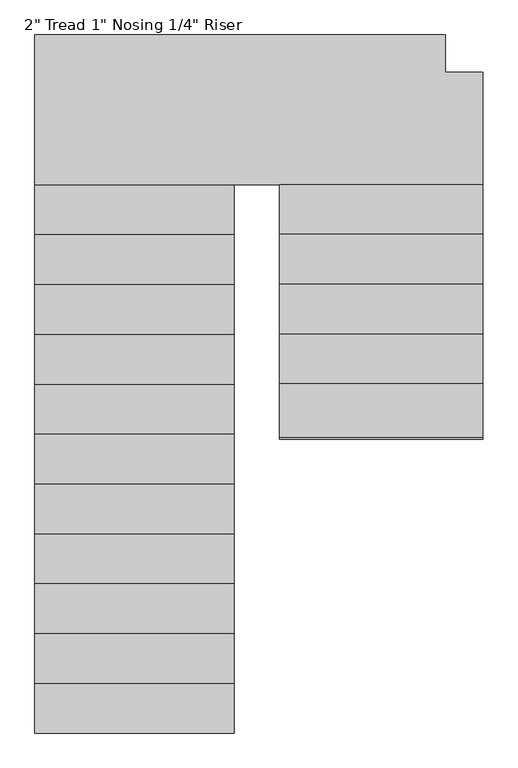
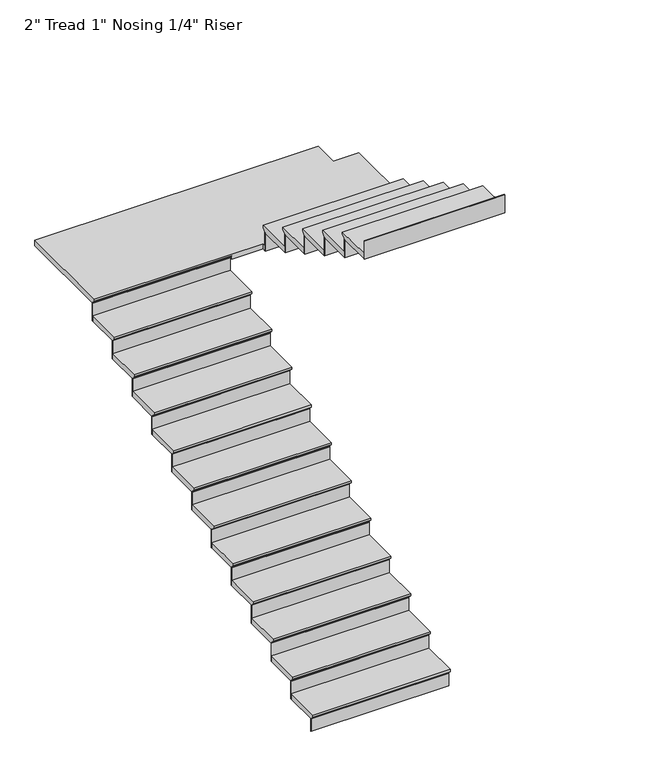
"""IFC4 building model written with IfcOpenShell, lengths in millimetres: stair flight geometry."""

from ifc_helpers import new_model, si_unit, origin, place, context, project, spatial, faceted_brep, source, transform, mapped, element, save


def stair_flight_d695bd93(model_context):
    return source(origin(), model_context, "Body", "Brep", [
        faceted_brep([(-1810.3456086, -4300.9794704, 3503.0833333), (-1810.3456086, -4300.9794704, 3522.1333333), (-3029.5456086, -4300.9794704, 3522.1333333), (-3029.5456086, -4300.9794704, 3503.0833333), (-1810.3456086, -4275.5794704, 3477.6833333), (-3029.5456086, -4275.5794704, 3477.6833333), (-1810.3456086, -3970.7794704, 3522.1333333), (-3029.5456086, -3970.7794704, 3522.1333333), (-3029.5456086, -4275.5794704, 3471.3333333), (-3029.5456086, -3970.7794704, 3471.3333333), (-1810.3456086, -3970.7794704, 3471.3333333), (-1810.3456086, -4275.5794704, 3471.3333333)], [[[0, 1, 2, 3]], [[4, 0, 3, 5]], [[2, 1, 6, 7]], [[8, 9, 10, 11]], [[2, 7, 9, 8, 5, 3]], [[8, 11, 4, 5]], [[6, 1, 0, 4, 11, 10]], [[7, 6, 10, 9]]]),
        faceted_brep([(-1810.3456086, -4275.5794704, 3471.3333333), (-1810.3456086, -4275.5794704, 3352.8), (-1810.3456086, -4269.2294704, 3352.8), (-1810.3456086, -4269.2294704, 3471.3333333), (-3029.5456086, -4275.5794704, 3471.3333333), (-3029.5456086, -4269.2294704, 3471.3333333), (-3029.5456086, -4269.2294704, 3352.8), (-3029.5456086, -4275.5794704, 3352.8)], [[[0, 1, 2, 3]], [[4, 5, 6, 7]], [[1, 0, 4, 7]], [[2, 1, 7, 6]], [[3, 2, 6, 5]], [[0, 3, 5, 4]]]),
        faceted_brep([(-1810.3456086, -3970.7794704, 3640.6666667), (-1810.3456086, -3970.7794704, 3471.3333333), (-1810.3456086, -3964.4294704, 3471.3333333), (-1810.3456086, -3964.4294704, 3640.6666667), (-3029.5456086, -3970.7794704, 3640.6666667), (-3029.5456086, -3964.4294704, 3640.6666667), (-3029.5456086, -3964.4294704, 3471.3333333), (-3029.5456086, -3970.7794704, 3471.3333333)], [[[0, 1, 2, 3]], [[4, 5, 6, 7]], [[1, 0, 4, 7]], [[2, 1, 7, 6]], [[3, 2, 6, 5]], [[0, 3, 5, 4]]]),
        faceted_brep([(-3029.5456086, -3996.1794704, 3691.4666667), (-1810.3456086, -3996.1794704, 3691.4666667), (-1810.3456086, -3665.9794704, 3691.4666667), (-3029.5456086, -3665.9794704, 3691.4666667), (-3029.5456086, -3970.7794704, 3640.6666667), (-3029.5456086, -3665.9794704, 3640.6666667), (-1810.3456086, -3665.9794704, 3640.6666667), (-1810.3456086, -3970.7794704, 3640.6666667), (-3029.5456086, -3970.7794704, 3647.0166667), (-3029.5456086, -3996.1794704, 3672.4166667), (-1810.3456086, -3970.7794704, 3647.0166667), (-1810.3456086, -3996.1794704, 3672.4166667)], [[[0, 1, 2, 3]], [[4, 5, 6, 7]], [[0, 3, 5, 4, 8, 9]], [[4, 7, 10, 8]], [[2, 1, 11, 10, 7, 6]], [[3, 2, 6, 5]], [[11, 1, 0, 9]], [[10, 11, 9, 8]]]),
        faceted_brep([(-1810.3456086, -3665.9794704, 3810.0), (-1810.3456086, -3665.9794704, 3640.6666667), (-1810.3456086, -3659.6294704, 3640.6666667), (-1810.3456086, -3659.6294704, 3810.0), (-3029.5456086, -3665.9794704, 3810.0), (-3029.5456086, -3659.6294704, 3810.0), (-3029.5456086, -3659.6294704, 3640.6666667), (-3029.5456086, -3665.9794704, 3640.6666667)], [[[0, 1, 2, 3]], [[4, 5, 6, 7]], [[1, 0, 4, 7]], [[2, 1, 7, 6]], [[3, 2, 6, 5]], [[0, 3, 5, 4]]]),
        faceted_brep([(-3029.5456086, -3691.3794704, 3860.8), (-1810.3456086, -3691.3794704, 3860.8), (-1810.3456086, -3361.1794704, 3860.8), (-3029.5456086, -3361.1794704, 3860.8), (-3029.5456086, -3665.9794704, 3810.0), (-3029.5456086, -3361.1794704, 3810.0), (-1810.3456086, -3361.1794704, 3810.0), (-1810.3456086, -3665.9794704, 3810.0), (-3029.5456086, -3665.9794704, 3816.35), (-3029.5456086, -3691.3794704, 3841.75), (-1810.3456086, -3665.9794704, 3816.35), (-1810.3456086, -3691.3794704, 3841.75)], [[[0, 1, 2, 3]], [[4, 5, 6, 7]], [[0, 3, 5, 4, 8, 9]], [[4, 7, 10, 8]], [[2, 1, 11, 10, 7, 6]], [[3, 2, 6, 5]], [[11, 1, 0, 9]], [[10, 11, 9, 8]]]),
        faceted_brep([(-1810.3456086, -3361.1794704, 3979.3333333), (-1810.3456086, -3361.1794704, 3810.0), (-1810.3456086, -3354.8294704, 3810.0), (-1810.3456086, -3354.8294704, 3979.3333333), (-3029.5456086, -3361.1794704, 3979.3333333), (-3029.5456086, -3354.8294704, 3979.3333333), (-3029.5456086, -3354.8294704, 3810.0), (-3029.5456086, -3361.1794704, 3810.0)], [[[0, 1, 2, 3]], [[4, 5, 6, 7]], [[1, 0, 4, 7]], [[2, 1, 7, 6]], [[3, 2, 6, 5]], [[0, 3, 5, 4]]]),
        faceted_brep([(-3029.5456086, -3386.5794704, 4030.1333333), (-1810.3456086, -3386.5794704, 4030.1333333), (-1810.3456086, -3056.3794704, 4030.1333333), (-3029.5456086, -3056.3794704, 4030.1333333), (-3029.5456086, -3361.1794704, 3979.3333333), (-3029.5456086, -3056.3794704, 3979.3333333), (-1810.3456086, -3056.3794704, 3979.3333333), (-1810.3456086, -3361.1794704, 3979.3333333), (-3029.5456086, -3361.1794704, 3985.6833333), (-3029.5456086, -3386.5794704, 4011.0833333), (-1810.3456086, -3361.1794704, 3985.6833333), (-1810.3456086, -3386.5794704, 4011.0833333)], [[[0, 1, 2, 3]], [[4, 5, 6, 7]], [[0, 3, 5, 4, 8, 9]], [[4, 7, 10, 8]], [[2, 1, 11, 10, 7, 6]], [[3, 2, 6, 5]], [[11, 1, 0, 9]], [[10, 11, 9, 8]]]),
        faceted_brep([(-1810.3456086, -3056.3794704, 4148.6666667), (-1810.3456086, -3056.3794704, 3979.3333333), (-1810.3456086, -3050.0294704, 3979.3333333), (-1810.3456086, -3050.0294704, 4148.6666667), (-3029.5456086, -3056.3794704, 4148.6666667), (-3029.5456086, -3050.0294704, 4148.6666667), (-3029.5456086, -3050.0294704, 3979.3333333), (-3029.5456086, -3056.3794704, 3979.3333333)], [[[0, 1, 2, 3]], [[4, 5, 6, 7]], [[1, 0, 4, 7]], [[2, 1, 7, 6]], [[3, 2, 6, 5]], [[0, 3, 5, 4]]]),
        faceted_brep([(-3029.5456086, -3081.7794704, 4199.4666667), (-1810.3456086, -3081.7794704, 4199.4666667), (-1810.3456086, -2751.5794704, 4199.4666667), (-3029.5456086, -2751.5794704, 4199.4666667), (-3029.5456086, -3056.3794704, 4148.6666667), (-3029.5456086, -2751.5794704, 4148.6666667), (-1810.3456086, -2751.5794704, 4148.6666667), (-1810.3456086, -3056.3794704, 4148.6666667), (-3029.5456086, -3056.3794704, 4155.0166667), (-3029.5456086, -3081.7794704, 4180.4166667), (-1810.3456086, -3056.3794704, 4155.0166667), (-1810.3456086, -3081.7794704, 4180.4166667)], [[[0, 1, 2, 3]], [[4, 5, 6, 7]], [[0, 3, 5, 4, 8, 9]], [[4, 7, 10, 8]], [[2, 1, 11, 10, 7, 6]], [[3, 2, 6, 5]], [[11, 1, 0, 9]], [[10, 11, 9, 8]]]),
        faceted_brep([(-1810.3456086, -2751.5794704, 4318.0), (-1810.3456086, -2751.5794704, 4148.6666667), (-1810.3456086, -2745.2294704, 4148.6666667), (-1810.3456086, -2745.2294704, 4318.0), (-3029.5456086, -2751.5794704, 4318.0), (-3029.5456086, -2745.2294704, 4318.0), (-3029.5456086, -2745.2294704, 4148.6666667), (-3029.5456086, -2751.5794704, 4148.6666667)], [[[0, 1, 2, 3]], [[4, 5, 6, 7]], [[1, 0, 4, 7]], [[2, 1, 7, 6]], [[3, 2, 6, 5]], [[0, 3, 5, 4]]]),
        faceted_brep([(-3029.5456086, -2776.9794704, 4368.8), (-1810.3456086, -2776.9794704, 4368.8), (-1810.3456086, -2446.7794704, 4368.8), (-3029.5456086, -2446.7794704, 4368.8), (-3029.5456086, -2751.5794704, 4318.0), (-3029.5456086, -2446.7794704, 4318.0), (-1810.3456086, -2446.7794704, 4318.0), (-1810.3456086, -2751.5794704, 4318.0), (-3029.5456086, -2751.5794704, 4324.35), (-3029.5456086, -2776.9794704, 4349.75), (-1810.3456086, -2751.5794704, 4324.35), (-1810.3456086, -2776.9794704, 4349.75)], [[[0, 1, 2, 3]], [[4, 5, 6, 7]], [[0, 3, 5, 4, 8, 9]], [[4, 7, 10, 8]], [[2, 1, 11, 10, 7, 6]], [[3, 2, 6, 5]], [[11, 1, 0, 9]], [[10, 11, 9, 8]]]),
        faceted_brep([(-1810.3456086, -2446.7794704, 4487.3333333), (-1810.3456086, -2446.7794704, 4318.0), (-1810.3456086, -2440.4294704, 4318.0), (-1810.3456086, -2440.4294704, 4487.3333333), (-3029.5456086, -2446.7794704, 4487.3333333), (-3029.5456086, -2440.4294704, 4487.3333333), (-3029.5456086, -2440.4294704, 4318.0), (-3029.5456086, -2446.7794704, 4318.0)], [[[0, 1, 2, 3]], [[4, 5, 6, 7]], [[1, 0, 4, 7]], [[2, 1, 7, 6]], [[3, 2, 6, 5]], [[0, 3, 5, 4]]]),
        faceted_brep([(-3029.5456086, -2472.1794704, 4538.1333333), (-1810.3456086, -2472.1794704, 4538.1333333), (-1810.3456086, -2141.9794704, 4538.1333333), (-3029.5456086, -2141.9794704, 4538.1333333), (-3029.5456086, -2446.7794704, 4487.3333333), (-3029.5456086, -2141.9794704, 4487.3333333), (-1810.3456086, -2141.9794704, 4487.3333333), (-1810.3456086, -2446.7794704, 4487.3333333), (-3029.5456086, -2446.7794704, 4493.6833333), (-3029.5456086, -2472.1794704, 4519.0833333), (-1810.3456086, -2446.7794704, 4493.6833333), (-1810.3456086, -2472.1794704, 4519.0833333)], [[[0, 1, 2, 3]], [[4, 5, 6, 7]], [[0, 3, 5, 4, 8, 9]], [[4, 7, 10, 8]], [[2, 1, 11, 10, 7, 6]], [[3, 2, 6, 5]], [[11, 1, 0, 9]], [[10, 11, 9, 8]]]),
        faceted_brep([(-1810.3456086, -2141.9794704, 4656.6666667), (-1810.3456086, -2141.9794704, 4487.3333333), (-1810.3456086, -2135.6294704, 4487.3333333), (-1810.3456086, -2135.6294704, 4656.6666667), (-3029.5456086, -2141.9794704, 4656.6666667), (-3029.5456086, -2135.6294704, 4656.6666667), (-3029.5456086, -2135.6294704, 4487.3333333), (-3029.5456086, -2141.9794704, 4487.3333333)], [[[0, 1, 2, 3]], [[4, 5, 6, 7]], [[1, 0, 4, 7]], [[2, 1, 7, 6]], [[3, 2, 6, 5]], [[0, 3, 5, 4]]]),
        faceted_brep([(-3029.5456086, -2167.3794704, 4707.4666667), (-1810.3456086, -2167.3794704, 4707.4666667), (-1810.3456086, -1837.1794704, 4707.4666667), (-3029.5456086, -1837.1794704, 4707.4666667), (-3029.5456086, -2141.9794704, 4656.6666667), (-3029.5456086, -1837.1794704, 4656.6666667), (-1810.3456086, -1837.1794704, 4656.6666667), (-1810.3456086, -2141.9794704, 4656.6666667), (-3029.5456086, -2141.9794704, 4663.0166667), (-3029.5456086, -2167.3794704, 4688.4166667), (-1810.3456086, -2141.9794704, 4663.0166667), (-1810.3456086, -2167.3794704, 4688.4166667)], [[[0, 1, 2, 3]], [[4, 5, 6, 7]], [[0, 3, 5, 4, 8, 9]], [[4, 7, 10, 8]], [[2, 1, 11, 10, 7, 6]], [[3, 2, 6, 5]], [[11, 1, 0, 9]], [[10, 11, 9, 8]]]),
        faceted_brep([(-1810.3456086, -1837.1794704, 4826.0), (-1810.3456086, -1837.1794704, 4656.6666667), (-1810.3456086, -1830.8294704, 4656.6666667), (-1810.3456086, -1830.8294704, 4826.0), (-3029.5456086, -1837.1794704, 4826.0), (-3029.5456086, -1830.8294704, 4826.0), (-3029.5456086, -1830.8294704, 4656.6666667), (-3029.5456086, -1837.1794704, 4656.6666667)], [[[0, 1, 2, 3]], [[4, 5, 6, 7]], [[1, 0, 4, 7]], [[2, 1, 7, 6]], [[3, 2, 6, 5]], [[0, 3, 5, 4]]]),
        faceted_brep([(-3029.5456086, -1862.5794704, 4876.8), (-1810.3456086, -1862.5794704, 4876.8), (-1810.3456086, -1532.3794704, 4876.8), (-3029.5456086, -1532.3794704, 4876.8), (-3029.5456086, -1837.1794704, 4826.0), (-3029.5456086, -1532.3794704, 4826.0), (-1810.3456086, -1532.3794704, 4826.0), (-1810.3456086, -1837.1794704, 4826.0), (-3029.5456086, -1837.1794704, 4832.35), (-3029.5456086, -1862.5794704, 4857.75), (-1810.3456086, -1837.1794704, 4832.35), (-1810.3456086, -1862.5794704, 4857.75)], [[[0, 1, 2, 3]], [[4, 5, 6, 7]], [[0, 3, 5, 4, 8, 9]], [[4, 7, 10, 8]], [[2, 1, 11, 10, 7, 6]], [[3, 2, 6, 5]], [[11, 1, 0, 9]], [[10, 11, 9, 8]]]),
        faceted_brep([(-1810.3456086, -1532.3794704, 4995.3333333), (-1810.3456086, -1532.3794704, 4826.0), (-1810.3456086, -1526.0294704, 4826.0), (-1810.3456086, -1526.0294704, 4995.3333333), (-3029.5456086, -1532.3794704, 4995.3333333), (-3029.5456086, -1526.0294704, 4995.3333333), (-3029.5456086, -1526.0294704, 4826.0), (-3029.5456086, -1532.3794704, 4826.0)], [[[0, 1, 2, 3]], [[4, 5, 6, 7]], [[1, 0, 4, 7]], [[2, 1, 7, 6]], [[3, 2, 6, 5]], [[0, 3, 5, 4]]]),
        faceted_brep([(-3029.5456086, -1557.7794704, 5046.1333333), (-1810.3456086, -1557.7794704, 5046.1333333), (-1810.3456086, -1227.5794704, 5046.1333333), (-3029.5456086, -1227.5794704, 5046.1333333), (-3029.5456086, -1532.3794704, 4995.3333333), (-3029.5456086, -1227.5794704, 4995.3333333), (-1810.3456086, -1227.5794704, 4995.3333333), (-1810.3456086, -1532.3794704, 4995.3333333), (-3029.5456086, -1532.3794704, 5001.6833333), (-3029.5456086, -1557.7794704, 5027.0833333), (-1810.3456086, -1532.3794704, 5001.6833333), (-1810.3456086, -1557.7794704, 5027.0833333)], [[[0, 1, 2, 3]], [[4, 5, 6, 7]], [[0, 3, 5, 4, 8, 9]], [[4, 7, 10, 8]], [[2, 1, 11, 10, 7, 6]], [[3, 2, 6, 5]], [[11, 1, 0, 9]], [[10, 11, 9, 8]]]),
        faceted_brep([(-1810.3456086, -1227.5794704, 5164.6666667), (-1810.3456086, -1227.5794704, 4995.3333333), (-1810.3456086, -1221.2294704, 4995.3333333), (-1810.3456086, -1221.2294704, 5164.6666667), (-3029.5456086, -1227.5794704, 5164.6666667), (-3029.5456086, -1221.2294704, 5164.6666667), (-3029.5456086, -1221.2294704, 4995.3333333), (-3029.5456086, -1227.5794704, 4995.3333333)], [[[0, 1, 2, 3]], [[4, 5, 6, 7]], [[1, 0, 4, 7]], [[2, 1, 7, 6]], [[3, 2, 6, 5]], [[0, 3, 5, 4]]]),
        faceted_brep([(-3029.5456086, -1252.9794704, 5215.4666667), (-1810.3456086, -1252.9794704, 5215.4666667), (-1810.3456086, -922.7794704, 5215.4666667), (-3029.5456086, -922.7794704, 5215.4666667), (-3029.5456086, -1227.5794704, 5164.6666667), (-3029.5456086, -922.7794704, 5164.6666667), (-1810.3456086, -922.7794704, 5164.6666667), (-1810.3456086, -1227.5794704, 5164.6666667), (-3029.5456086, -1227.5794704, 5171.0166667), (-3029.5456086, -1252.9794704, 5196.4166667), (-1810.3456086, -1227.5794704, 5171.0166667), (-1810.3456086, -1252.9794704, 5196.4166667)], [[[0, 1, 2, 3]], [[4, 5, 6, 7]], [[0, 3, 5, 4, 8, 9]], [[4, 7, 10, 8]], [[2, 1, 11, 10, 7, 6]], [[3, 2, 6, 5]], [[11, 1, 0, 9]], [[10, 11, 9, 8]]]),
        faceted_brep([(-1810.3456086, -922.7794704, 5334.0), (-1810.3456086, -922.7794704, 5164.6666667), (-1810.3456086, -916.4294704, 5164.6666667), (-1810.3456086, -916.4294704, 5334.0), (-3029.5456086, -922.7794704, 5334.0), (-3029.5456086, -916.4294704, 5334.0), (-3029.5456086, -916.4294704, 5164.6666667), (-3029.5456086, -922.7794704, 5164.6666667)], [[[0, 1, 2, 3]], [[4, 5, 6, 7]], [[1, 0, 4, 7]], [[2, 1, 7, 6]], [[3, 2, 6, 5]], [[0, 3, 5, 4]]]),
        faceted_brep([(-289.8083398, -973.5794704, 5384.8), (-289.8083398, -262.3794704, 5384.8), (-518.4083398, -262.3794704, 5384.8), (-518.4083398, -33.7794704, 5384.8), (-3029.5456086, -33.7794704, 5384.8), (-3029.5456086, -948.1794704, 5384.8), (-1534.4083398, -948.1794704, 5384.8), (-1534.4083398, -973.5794704, 5384.8), (-289.8083398, -262.3794704, 5334.0), (-289.8083398, -973.5794704, 5334.0), (-1534.4083398, -973.5794704, 5334.0), (-1534.4083398, -948.1794704, 5334.0), (-1810.3456086, -948.1794704, 5334.0), (-1810.3456086, -922.7794704, 5334.0), (-3029.5456086, -922.7794704, 5334.0), (-3029.5456086, -33.7794704, 5334.0), (-518.4083398, -33.7794704, 5334.0), (-518.4083398, -262.3794704, 5334.0), (-3029.5456086, -922.7794704, 5340.35), (-3029.5456086, -948.1794704, 5365.75), (-1810.3456086, -922.7794704, 5340.35), (-1810.3456086, -948.1794704, 5365.75)], [[[0, 1, 2, 3, 4, 5, 6, 7]], [[8, 9, 10, 11, 12, 13, 14, 15, 16, 17]], [[1, 0, 9, 8]], [[2, 1, 8, 17]], [[3, 2, 17, 16]], [[4, 3, 16, 15]], [[5, 4, 15, 14, 18, 19]], [[14, 13, 20, 18]], [[13, 12, 21, 20]], [[6, 5, 19, 21, 12, 11]], [[7, 6, 11, 10]], [[0, 7, 10, 9]], [[19, 18, 20, 21]]]),
        faceted_brep([(-1534.4083398, -973.5794704, 5503.3333333), (-1534.4083398, -973.5794704, 5334.0), (-1534.4083398, -979.9294704, 5334.0), (-1534.4083398, -979.9294704, 5503.3333333), (-289.8083398, -973.5794704, 5503.3333333), (-289.8083398, -979.9294704, 5503.3333333), (-289.8083398, -979.9294704, 5334.0), (-289.8083398, -973.5794704, 5334.0)], [[[0, 1, 2, 3]], [[4, 5, 6, 7]], [[1, 0, 4, 7]], [[2, 1, 7, 6]], [[3, 2, 6, 5]], [[0, 3, 5, 4]]]),
        faceted_brep([(-289.8083398, -948.1794704, 5554.1333333), (-1534.4083398, -948.1794704, 5554.1333333), (-1534.4083398, -1278.3794704, 5554.1333333), (-289.8083398, -1278.3794704, 5554.1333333), (-289.8083398, -973.5794704, 5503.3333333), (-289.8083398, -1278.3794704, 5503.3333333), (-1534.4083398, -1278.3794704, 5503.3333333), (-1534.4083398, -973.5794704, 5503.3333333), (-289.8083398, -973.5794704, 5509.6833333), (-289.8083398, -948.1794704, 5535.0833333), (-1534.4083398, -973.5794704, 5509.6833333), (-1534.4083398, -948.1794704, 5535.0833333)], [[[0, 1, 2, 3]], [[4, 5, 6, 7]], [[0, 3, 5, 4, 8, 9]], [[4, 7, 10, 8]], [[2, 1, 11, 10, 7, 6]], [[3, 2, 6, 5]], [[11, 1, 0, 9]], [[10, 11, 9, 8]]]),
        faceted_brep([(-1534.4083398, -1278.3794704, 5672.6666667), (-1534.4083398, -1278.3794704, 5503.3333333), (-1534.4083398, -1284.7294704, 5503.3333333), (-1534.4083398, -1284.7294704, 5672.6666667), (-289.8083398, -1278.3794704, 5672.6666667), (-289.8083398, -1284.7294704, 5672.6666667), (-289.8083398, -1284.7294704, 5503.3333333), (-289.8083398, -1278.3794704, 5503.3333333)], [[[0, 1, 2, 3]], [[4, 5, 6, 7]], [[1, 0, 4, 7]], [[2, 1, 7, 6]], [[3, 2, 6, 5]], [[0, 3, 5, 4]]]),
        faceted_brep([(-289.8083398, -1252.9794704, 5723.4666667), (-1534.4083398, -1252.9794704, 5723.4666667), (-1534.4083398, -1583.1794704, 5723.4666667), (-289.8083398, -1583.1794704, 5723.4666667), (-289.8083398, -1278.3794704, 5672.6666667), (-289.8083398, -1583.1794704, 5672.6666667), (-1534.4083398, -1583.1794704, 5672.6666667), (-1534.4083398, -1278.3794704, 5672.6666667), (-289.8083398, -1278.3794704, 5679.0166667), (-289.8083398, -1252.9794704, 5704.4166667), (-1534.4083398, -1278.3794704, 5679.0166667), (-1534.4083398, -1252.9794704, 5704.4166667)], [[[0, 1, 2, 3]], [[4, 5, 6, 7]], [[0, 3, 5, 4, 8, 9]], [[4, 7, 10, 8]], [[2, 1, 11, 10, 7, 6]], [[3, 2, 6, 5]], [[11, 1, 0, 9]], [[10, 11, 9, 8]]]),
        faceted_brep([(-1534.4083398, -1583.1794704, 5842.0), (-1534.4083398, -1583.1794704, 5672.6666667), (-1534.4083398, -1589.5294704, 5672.6666667), (-1534.4083398, -1589.5294704, 5842.0), (-289.8083398, -1583.1794704, 5842.0), (-289.8083398, -1589.5294704, 5842.0), (-289.8083398, -1589.5294704, 5672.6666667), (-289.8083398, -1583.1794704, 5672.6666667)], [[[0, 1, 2, 3]], [[4, 5, 6, 7]], [[1, 0, 4, 7]], [[2, 1, 7, 6]], [[3, 2, 6, 5]], [[0, 3, 5, 4]]]),
        faceted_brep([(-289.8083398, -1557.7794704, 5892.8), (-1534.4083398, -1557.7794704, 5892.8), (-1534.4083398, -1887.9794704, 5892.8), (-289.8083398, -1887.9794704, 5892.8), (-289.8083398, -1583.1794704, 5842.0), (-289.8083398, -1887.9794704, 5842.0), (-1534.4083398, -1887.9794704, 5842.0), (-1534.4083398, -1583.1794704, 5842.0), (-289.8083398, -1583.1794704, 5848.35), (-289.8083398, -1557.7794704, 5873.75), (-1534.4083398, -1583.1794704, 5848.35), (-1534.4083398, -1557.7794704, 5873.75)], [[[0, 1, 2, 3]], [[4, 5, 6, 7]], [[0, 3, 5, 4, 8, 9]], [[4, 7, 10, 8]], [[2, 1, 11, 10, 7, 6]], [[3, 2, 6, 5]], [[11, 1, 0, 9]], [[10, 11, 9, 8]]]),
        faceted_brep([(-1534.4083398, -1887.9794704, 6011.3333333), (-1534.4083398, -1887.9794704, 5842.0), (-1534.4083398, -1894.3294704, 5842.0), (-1534.4083398, -1894.3294704, 6011.3333333), (-289.8083398, -1887.9794704, 6011.3333333), (-289.8083398, -1894.3294704, 6011.3333333), (-289.8083398, -1894.3294704, 5842.0), (-289.8083398, -1887.9794704, 5842.0)], [[[0, 1, 2, 3]], [[4, 5, 6, 7]], [[1, 0, 4, 7]], [[2, 1, 7, 6]], [[3, 2, 6, 5]], [[0, 3, 5, 4]]]),
        faceted_brep([(-289.8083398, -1862.5794704, 6062.1333333), (-1534.4083398, -1862.5794704, 6062.1333333), (-1534.4083398, -2192.7794704, 6062.1333333), (-289.8083398, -2192.7794704, 6062.1333333), (-289.8083398, -1887.9794704, 6011.3333333), (-289.8083398, -2192.7794704, 6011.3333333), (-1534.4083398, -2192.7794704, 6011.3333333), (-1534.4083398, -1887.9794704, 6011.3333333), (-289.8083398, -1887.9794704, 6017.6833333), (-289.8083398, -1862.5794704, 6043.0833333), (-1534.4083398, -1887.9794704, 6017.6833333), (-1534.4083398, -1862.5794704, 6043.0833333)], [[[0, 1, 2, 3]], [[4, 5, 6, 7]], [[0, 3, 5, 4, 8, 9]], [[4, 7, 10, 8]], [[2, 1, 11, 10, 7, 6]], [[3, 2, 6, 5]], [[11, 1, 0, 9]], [[10, 11, 9, 8]]]),
        faceted_brep([(-1534.4083398, -2192.7794704, 6180.6666667), (-1534.4083398, -2192.7794704, 6011.3333333), (-1534.4083398, -2199.1294704, 6011.3333333), (-1534.4083398, -2199.1294704, 6180.6666667), (-289.8083398, -2192.7794704, 6180.6666667), (-289.8083398, -2199.1294704, 6180.6666667), (-289.8083398, -2199.1294704, 6011.3333333), (-289.8083398, -2192.7794704, 6011.3333333)], [[[0, 1, 2, 3]], [[4, 5, 6, 7]], [[1, 0, 4, 7]], [[2, 1, 7, 6]], [[3, 2, 6, 5]], [[0, 3, 5, 4]]]),
        faceted_brep([(-1534.4083398, -2497.5794704, 6350.0), (-1534.4083398, -2497.5794704, 6180.6666667), (-1534.4083398, -2503.9294704, 6180.6666667), (-1534.4083398, -2503.9294704, 6350.0), (-289.8083398, -2497.5794704, 6350.0), (-289.8083398, -2503.9294704, 6350.0), (-289.8083398, -2503.9294704, 6180.6666667), (-289.8083398, -2497.5794704, 6180.6666667)], [[[0, 1, 2, 3]], [[4, 5, 6, 7]], [[1, 0, 4, 7]], [[2, 1, 7, 6]], [[3, 2, 6, 5]], [[0, 3, 5, 4]]]),
        faceted_brep([(-289.8083398, -2167.3794704, 6231.4666667), (-1534.4083398, -2167.3794704, 6231.4666667), (-1534.4083398, -2497.5794704, 6231.4666667), (-289.8083398, -2497.5794704, 6231.4666667), (-289.8083398, -2192.7794704, 6180.6666667), (-289.8083398, -2497.5794704, 6180.6666667), (-1534.4083398, -2497.5794704, 6180.6666667), (-1534.4083398, -2192.7794704, 6180.6666667), (-289.8083398, -2192.7794704, 6187.0166667), (-289.8083398, -2167.3794704, 6212.4166667), (-1534.4083398, -2192.7794704, 6187.0166667), (-1534.4083398, -2167.3794704, 6212.4166667)], [[[0, 1, 2, 3]], [[4, 5, 6, 7]], [[0, 3, 5, 4, 8, 9]], [[4, 7, 10, 8]], [[2, 1, 11, 10, 7, 6]], [[3, 2, 6, 5]], [[11, 1, 0, 9]], [[10, 11, 9, 8]]]),
    ])


if __name__ == "__main__":
    model = new_model("IFC4")
    model_context = context("Model", 3, world=origin())
    ifc_project = project(units=[si_unit("LENGTHUNIT", "METRE", prefix="MILLI")], contexts=[model_context])
    site = spatial("IfcSite", under=ifc_project)
    building = spatial("IfcBuilding", under=site)
    placement = place(None, origin())
    stair_flight_shape = stair_flight_d695bd93(model_context)
    element("IfcStairFlight", 1, ObjectType="2\" Tread 1\" Nosing 1/4\" Riser", at=placement, inside=building, context=model_context, shape_type="MappedRepresentation", body=[
        mapped(stair_flight_shape, transform((0.0, 0.0, 0.0), x_axis=(1.0, 0.0, 0.0), y_axis=(0.0, 1.0, 0.0), z_axis=(0.0, 0.0, 1.0))),
    ])
    save(model, "model.ifc")
